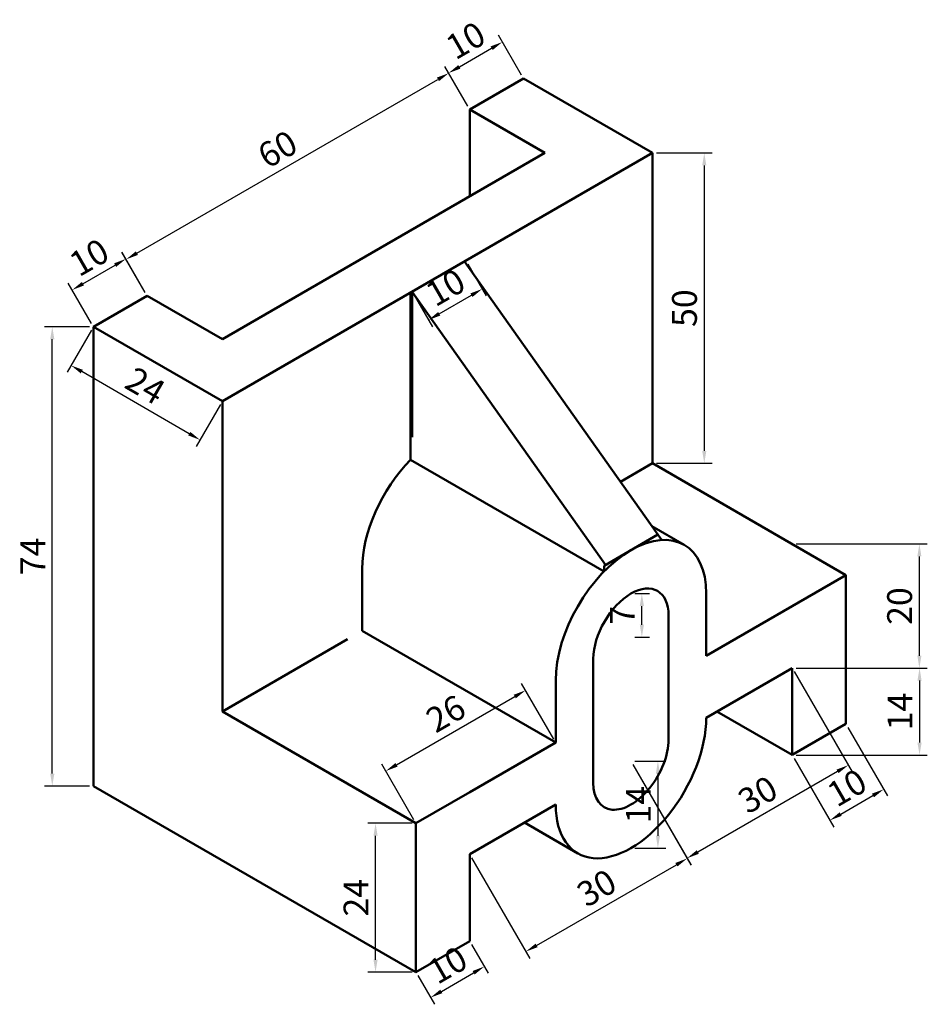
# Model space of a CAD drawing. Units: millimetres. Extents: x 109 to 256, y 55 to 213.
import ezdxf

# ---------------------------------------------------------------- set-up
doc = ezdxf.new("R2010")
doc.units = ezdxf.units.MM
doc.layers.add('M-DIMS', color=2, linetype='Continuous', lineweight=25)
doc.layers.add('M-OUTL', color=7, linetype='Continuous', lineweight=50)
doc.styles.get("Standard").update_dxf_attribs({"font": 'arial.ttf'})
doc.dimstyles.new('ISO-25', dxfattribs={"dimtxt": 4, "dimasz": 2, "dimexe": 1.25, "dimexo": 0.625, "dimtad": 1, "dimtxsty": 'Standard', "dimcen": 2.5, "dimadec": 0, "dimazin": 0, "dimtfac": 1, "dimtmove": 0, "dimatfit": 3, "dimfxl": 1, "dimarcsym": 0})

# ---------------------------------------------------------------- blocks, each defined once
blk = doc.blocks.new('*D1')
at = {"layer": 'Defpoints', "color": 0, "transparency": 16777216}
for p in [(121.32, 163.94), (117.73, 157.71), (142.11, 151.94)]:
    blk.add_point(p, dxfattribs=at)
at = {"layer": 'M-DIMS', "color": 0, "lineweight": -2, "transparency": 16777216}
for p, q in [((121.01, 163.4), (117.1, 156.63)), ((136.78, 146.71), (119.46, 156.71)), ((141.8, 151.4), (137.89, 144.63))]:
    blk.add_line(p, q, dxfattribs=at)
at = {"layer": 'M-DIMS', "color": 0, "transparency": 16777216}
for points in [[(119.63, 157), (119.29, 156.43), (117.73, 157.71)], [(136.95, 147), (136.61, 146.43), (138.51, 145.71)]]:
    blk.add_solid(points, dxfattribs=at)
at = {"layer": 'M-DIMS', "color": 0, "transparency": 16777216, "insert": (129.44, 154), "char_height": 4, "attachment_point": 5, "rotation": 330}
blk.add_mtext('24', dxfattribs=at)
blk = doc.blocks.new('*D2')
at = {"layer": 'Defpoints', "color": 0, "transparency": 16777216}
for p in [(126.56, 174.87), (129.98, 168.94), (121.32, 163.94)]:
    blk.add_point(p, dxfattribs=at)
at = {"layer": 'M-DIMS', "color": 0, "lineweight": -2, "transparency": 16777216}
for p, q in [((129.67, 169.48), (125.93, 175.96)), ((119.63, 170.87), (124.83, 173.87)), ((121.01, 164.48), (117.27, 170.96))]:
    blk.add_line(p, q, dxfattribs=at)
at = {"layer": 'M-DIMS', "color": 0, "transparency": 16777216}
for points in [[(124.66, 174.16), (124.99, 173.59), (126.56, 174.87)], [(119.47, 171.16), (119.8, 170.59), (117.9, 169.87)]]:
    blk.add_solid(points, dxfattribs=at)
at = {"layer": 'M-DIMS', "color": 0, "transparency": 16777216, "insert": (120.9, 174.68), "char_height": 4, "attachment_point": 5, "rotation": 30}
blk.add_mtext('10', dxfattribs=at)
blk = doc.blocks.new('*D3')
at = {"layer": 'Defpoints', "color": 0, "transparency": 16777216}
for p in [(178.56, 204.8), (181.95, 198.94), (129.98, 168.94)]:
    blk.add_point(p, dxfattribs=at)
at = {"layer": 'M-DIMS', "color": 0, "lineweight": -2, "transparency": 16777216}
for p, q in [((181.63, 199.48), (177.94, 205.88)), ((128.33, 175.8), (176.83, 203.8)), ((129.67, 169.48), (125.98, 175.88))]:
    blk.add_line(p, q, dxfattribs=at)
at = {"layer": 'M-DIMS', "color": 0, "transparency": 16777216}
for points in [[(176.67, 204.09), (177, 203.51), (178.56, 204.8)], [(128.17, 176.09), (128.5, 175.51), (126.6, 174.8)]]:
    blk.add_solid(points, dxfattribs=at)
at = {"layer": 'M-DIMS', "color": 0, "transparency": 16777216, "insert": (151.25, 192.11), "char_height": 4, "attachment_point": 5, "rotation": 30}
blk.add_mtext('60', dxfattribs=at)
blk = doc.blocks.new('*D4')
at = {"layer": 'Defpoints', "color": 0, "transparency": 16777216}
for p in [(187.21, 209.82), (190.61, 203.94), (181.95, 198.94)]:
    blk.add_point(p, dxfattribs=at)
at = {"layer": 'M-DIMS', "color": 0, "lineweight": -2, "transparency": 16777216}
for p, q in [((190.29, 204.48), (186.59, 210.9)), ((180.29, 205.82), (185.48, 208.82)), ((181.63, 199.48), (177.93, 205.9))]:
    blk.add_line(p, q, dxfattribs=at)
at = {"layer": 'M-DIMS', "color": 0, "transparency": 16777216}
for points in [[(185.31, 209.11), (185.65, 208.53), (187.21, 209.82)], [(180.12, 206.11), (180.45, 205.53), (178.55, 204.82)]]:
    blk.add_solid(points, dxfattribs=at)
at = {"layer": 'M-DIMS', "color": 0, "transparency": 16777216, "insert": (181.55, 209.63), "char_height": 4, "attachment_point": 5, "rotation": 30}
blk.add_mtext('10', dxfattribs=at)
blk = doc.blocks.new('*D5')
at = {"layer": 'Defpoints', "color": 0, "transparency": 16777216}
for p in [(211.39, 191.94), (211.39, 141.94), (219.74, 141.94)]:
    blk.add_point(p, dxfattribs=at)
at = {"layer": 'M-DIMS', "color": 0, "lineweight": -2, "transparency": 16777216}
for p, q in [((212.02, 191.94), (220.99, 191.94)), ((219.74, 189.94), (219.74, 143.94)), ((212.02, 141.94), (220.99, 141.94))]:
    blk.add_line(p, q, dxfattribs=at)
at = {"layer": 'M-DIMS', "color": 0, "transparency": 16777216}
for points in [[(219.4, 189.94), (220.07, 189.94), (219.74, 191.94)], [(219.4, 143.94), (220.07, 143.94), (219.74, 141.94)]]:
    blk.add_solid(points, dxfattribs=at)
at = {"layer": 'M-DIMS', "color": 0, "transparency": 16777216, "insert": (217.07, 166.94), "char_height": 4, "attachment_point": 5, "rotation": 90}
blk.add_mtext('50', dxfattribs=at)
blk = doc.blocks.new('*D6')
at = {"layer": 'Defpoints', "color": 0, "transparency": 16777216}
for p in [(233.91, 128.94), (254.39, 128.94), (233.91, 108.94)]:
    blk.add_point(p, dxfattribs=at)
at = {"layer": 'M-DIMS', "color": 0, "lineweight": -2, "transparency": 16777216}
for p, q in [((234.53, 128.94), (255.64, 128.94)), ((254.39, 110.94), (254.39, 126.94)), ((234.53, 108.94), (255.64, 108.94))]:
    blk.add_line(p, q, dxfattribs=at)
at = {"layer": 'M-DIMS', "color": 0, "transparency": 16777216}
for points in [[(254.06, 126.94), (254.72, 126.94), (254.39, 128.94)], [(254.06, 110.94), (254.72, 110.94), (254.39, 108.94)]]:
    blk.add_solid(points, dxfattribs=at)
at = {"layer": 'M-DIMS', "color": 0, "transparency": 16777216, "insert": (251.72, 118.94), "char_height": 4, "attachment_point": 5, "rotation": 90}
blk.add_mtext('20', dxfattribs=at)
blk = doc.blocks.new('*D7')
at = {"layer": 'Defpoints', "color": 0, "transparency": 16777216}
for p in [(233.91, 108.94), (233.91, 94.94), (254.42, 94.94)]:
    blk.add_point(p, dxfattribs=at)
at = {"layer": 'M-DIMS', "color": 0, "lineweight": -2, "transparency": 16777216}
for p, q in [((234.53, 108.94), (255.67, 108.94)), ((254.42, 106.94), (254.42, 96.94)), ((234.53, 94.94), (255.67, 94.94))]:
    blk.add_line(p, q, dxfattribs=at)
at = {"layer": 'M-DIMS', "color": 0, "transparency": 16777216}
for points in [[(254.08, 106.94), (254.75, 106.94), (254.42, 108.94)], [(254.08, 96.94), (254.75, 96.94), (254.42, 94.94)]]:
    blk.add_solid(points, dxfattribs=at)
at = {"layer": 'M-DIMS', "color": 0, "transparency": 16777216, "insert": (251.78, 101.94), "char_height": 4, "attachment_point": 5, "rotation": 90}
blk.add_mtext('14', dxfattribs=at)
blk = doc.blocks.new('*D8')
at = {"layer": 'Defpoints', "color": 0, "transparency": 16777216}
for p in [(166.78, 83.94), (173.29, 83.94), (173.29, 59.94)]:
    blk.add_point(p, dxfattribs=at)
at = {"layer": 'M-DIMS', "color": 0, "lineweight": -2, "transparency": 16777216}
for p, q in [((172.66, 83.94), (165.53, 83.94)), ((166.78, 61.94), (166.78, 81.94)), ((172.66, 59.94), (165.53, 59.94))]:
    blk.add_line(p, q, dxfattribs=at)
at = {"layer": 'M-DIMS', "color": 0, "transparency": 16777216}
for points in [[(166.45, 81.94), (167.11, 81.94), (166.78, 83.94)], [(166.45, 61.94), (167.11, 61.94), (166.78, 59.94)]]:
    blk.add_solid(points, dxfattribs=at)
at = {"layer": 'M-DIMS', "color": 0, "transparency": 16777216, "insert": (164.15, 71.94), "char_height": 4, "attachment_point": 5, "rotation": 90}
blk.add_mtext('24', dxfattribs=at)
blk = doc.blocks.new('*D9')
at = {"layer": 'Defpoints', "color": 0, "transparency": 16777216}
for p in [(181.95, 64.94), (184.31, 60.86), (173.29, 59.94)]:
    blk.add_point(p, dxfattribs=at)
at = {"layer": 'M-DIMS', "color": 0, "lineweight": -2, "transparency": 16777216}
for p, q in [((182.26, 64.4), (184.93, 59.77)), ((173.6, 59.4), (176.27, 54.77)), ((177.38, 56.86), (182.57, 59.86))]:
    blk.add_line(p, q, dxfattribs=at)
at = {"layer": 'M-DIMS', "color": 0, "transparency": 16777216}
for points in [[(182.41, 60.14), (182.74, 59.57), (184.31, 60.86)], [(177.21, 57.14), (177.54, 56.57), (175.65, 55.86)]]:
    blk.add_solid(points, dxfattribs=at)
at = {"layer": 'M-DIMS', "color": 0, "transparency": 16777216, "insert": (178.64, 60.67), "char_height": 4, "attachment_point": 5, "rotation": 30}
blk.add_mtext('10', dxfattribs=at)
blk = doc.blocks.new('*D10')
at = {"layer": 'Defpoints', "color": 0, "transparency": 16777216}
for p in [(207.93, 93.94), (181.95, 78.94), (216.98, 78.27)]:
    blk.add_point(p, dxfattribs=at)
at = {"layer": 'M-DIMS', "color": 0, "lineweight": -2, "transparency": 16777216}
for p, q in [((208.24, 93.4), (217.6, 77.18)), ((182.26, 78.4), (191.62, 62.18)), ((192.73, 64.27), (215.25, 77.27))]:
    blk.add_line(p, q, dxfattribs=at)
at = {"layer": 'M-DIMS', "color": 0, "transparency": 16777216}
for points in [[(215.08, 77.55), (215.41, 76.98), (216.98, 78.27)], [(192.56, 64.55), (192.9, 63.98), (191, 63.27)]]:
    blk.add_solid(points, dxfattribs=at)
at = {"layer": 'M-DIMS', "color": 0, "transparency": 16777216, "insert": (202.65, 73.08), "char_height": 4, "attachment_point": 5, "rotation": 30}
blk.add_mtext('30', dxfattribs=at)
blk = doc.blocks.new('*D11')
at = {"layer": 'Defpoints', "color": 0, "transparency": 16777216}
for p in [(233.91, 108.94), (207.93, 93.94), (216.96, 78.3)]:
    blk.add_point(p, dxfattribs=at)
at = {"layer": 'M-DIMS', "color": 0, "lineweight": -2, "transparency": 16777216}
for p, q in [((234.22, 108.4), (243.56, 92.22)), ((208.24, 93.4), (217.58, 77.22)), ((241.2, 92.3), (218.69, 79.3))]:
    blk.add_line(p, q, dxfattribs=at)
at = {"layer": 'M-DIMS', "color": 0, "transparency": 16777216}
for points in [[(241.04, 92.59), (241.37, 92.02), (242.94, 93.3)], [(218.52, 79.59), (218.85, 79.02), (216.96, 78.3)]]:
    blk.add_solid(points, dxfattribs=at)
at = {"layer": 'M-DIMS', "color": 0, "transparency": 16777216, "insert": (228.61, 88.12), "char_height": 4, "attachment_point": 5, "rotation": 30}
blk.add_mtext('30', dxfattribs=at)
blk = doc.blocks.new('*D12')
at = {"layer": 'Defpoints', "color": 0, "transparency": 16777216}
for p in [(242.57, 99.94), (233.91, 94.94), (248.64, 89.42)]:
    blk.add_point(p, dxfattribs=at)
at = {"layer": 'M-DIMS', "color": 0, "lineweight": -2, "transparency": 16777216}
for p, q in [((242.88, 99.4), (249.27, 88.34)), ((234.22, 94.4), (240.61, 83.34)), ((241.72, 85.42), (246.91, 88.42))]:
    blk.add_line(p, q, dxfattribs=at)
at = {"layer": 'M-DIMS', "color": 0, "transparency": 16777216}
for points in [[(246.74, 88.71), (247.08, 88.13), (248.64, 89.42)], [(241.55, 85.71), (241.88, 85.13), (239.98, 84.42)]]:
    blk.add_solid(points, dxfattribs=at)
at = {"layer": 'M-DIMS', "color": 0, "transparency": 16777216, "insert": (242.98, 89.23), "char_height": 4, "attachment_point": 5, "rotation": 30}
blk.add_mtext('10', dxfattribs=at)
blk = doc.blocks.new('*D13')
at = {"layer": 'Defpoints', "color": 0, "transparency": 16777216}
for p in [(207.93, 93.94), (207.93, 79.94), (212.27, 79.94)]:
    blk.add_point(p, dxfattribs=at)
at = {"layer": 'M-DIMS', "color": 0, "lineweight": -2, "transparency": 16777216}
for p, q in [((208.55, 93.94), (213.52, 93.94)), ((212.27, 91.94), (212.27, 81.94)), ((208.55, 79.94), (213.52, 79.94))]:
    blk.add_line(p, q, dxfattribs=at)
at = {"layer": 'M-DIMS', "color": 0, "transparency": 16777216}
for points in [[(211.94, 91.94), (212.61, 91.94), (212.27, 93.94)], [(211.94, 81.94), (212.61, 81.94), (212.27, 79.94)]]:
    blk.add_solid(points, dxfattribs=at)
at = {"layer": 'M-DIMS', "color": 0, "transparency": 16777216, "insert": (209.64, 86.94), "char_height": 4, "attachment_point": 5, "rotation": 90}
blk.add_mtext('14', dxfattribs=at)
blk = doc.blocks.new('*D14')
at = {"layer": 'Defpoints', "color": 0, "transparency": 16777216}
for p in [(207.93, 120.94), (209.68, 120.94), (207.93, 113.94)]:
    blk.add_point(p, dxfattribs=at)
at = {"layer": 'M-DIMS', "color": 0, "lineweight": -2, "transparency": 16777216}
for p, q in [((208.55, 120.94), (210.93, 120.94)), ((209.68, 115.94), (209.68, 118.94)), ((208.55, 113.94), (210.93, 113.94))]:
    blk.add_line(p, q, dxfattribs=at)
at = {"layer": 'M-DIMS', "color": 0, "transparency": 16777216}
for points in [[(209.35, 118.94), (210.02, 118.94), (209.68, 120.94)], [(209.35, 115.94), (210.02, 115.94), (209.68, 113.94)]]:
    blk.add_solid(points, dxfattribs=at)
at = {"layer": 'M-DIMS', "color": 0, "transparency": 16777216, "insert": (207.06, 117.44), "char_height": 4, "attachment_point": 5, "rotation": 90}
blk.add_mtext('7', dxfattribs=at)
blk = doc.blocks.new('*D15')
at = {"layer": 'Defpoints', "color": 0, "transparency": 16777216}
for p in [(181.33, 174.59), (183.96, 170.03), (172.67, 169.59)]:
    blk.add_point(p, dxfattribs=at)
at = {"layer": 'M-DIMS', "color": 0, "lineweight": -2, "transparency": 16777216}
for p, q in [((181.64, 174.05), (184.59, 168.95)), ((172.98, 169.05), (175.93, 163.95)), ((177.03, 166.03), (182.23, 169.03))]:
    blk.add_line(p, q, dxfattribs=at)
at = {"layer": 'M-DIMS', "color": 0, "transparency": 16777216}
for points in [[(182.06, 169.32), (182.4, 168.74), (183.96, 170.03)], [(176.87, 166.32), (177.2, 165.74), (175.3, 165.03)]]:
    blk.add_solid(points, dxfattribs=at)
at = {"layer": 'M-DIMS', "color": 0, "transparency": 16777216, "insert": (178.3, 169.84), "char_height": 4, "attachment_point": 5, "rotation": 30}
blk.add_mtext('10', dxfattribs=at)
blk = doc.blocks.new('*D16')
at = {"layer": 'Defpoints', "color": 0, "transparency": 16777216}
for p in [(190.94, 105.36), (195.8, 96.94), (173.29, 83.94)]:
    blk.add_point(p, dxfattribs=at)
at = {"layer": 'M-DIMS', "color": 0, "lineweight": -2, "transparency": 16777216}
for p, q in [((195.49, 97.48), (190.32, 106.44)), ((170.16, 93.36), (189.21, 104.36)), ((172.97, 84.48), (167.8, 93.44))]:
    blk.add_line(p, q, dxfattribs=at)
at = {"layer": 'M-DIMS', "color": 0, "transparency": 16777216}
for points in [[(189.05, 104.65), (189.38, 104.07), (190.94, 105.36)], [(169.99, 93.65), (170.33, 93.07), (168.43, 92.36)]]:
    blk.add_solid(points, dxfattribs=at)
at = {"layer": 'M-DIMS', "color": 0, "transparency": 16777216, "insert": (178.35, 101.17), "char_height": 4, "attachment_point": 5, "rotation": 30}
blk.add_mtext('26', dxfattribs=at)
blk = doc.blocks.new('*D17')
at = {"layer": 'Defpoints', "color": 0, "transparency": 16777216}
for p in [(114.7, 163.94), (121.32, 163.94), (121.32, 89.94)]:
    blk.add_point(p, dxfattribs=at)
at = {"layer": 'M-DIMS', "color": 0, "lineweight": -2, "transparency": 16777216}
for p, q in [((120.7, 163.94), (113.45, 163.94)), ((114.7, 91.94), (114.7, 161.94)), ((120.7, 89.94), (113.45, 89.94))]:
    blk.add_line(p, q, dxfattribs=at)
at = {"layer": 'M-DIMS', "color": 0, "transparency": 16777216}
for points in [[(114.37, 161.94), (115.04, 161.94), (114.7, 163.94)], [(114.37, 91.94), (115.04, 91.94), (114.7, 89.94)]]:
    blk.add_solid(points, dxfattribs=at)
at = {"layer": 'M-DIMS', "color": 0, "transparency": 16777216, "insert": (112.08, 126.94), "char_height": 4, "attachment_point": 5, "rotation": 90}
blk.add_mtext('74', dxfattribs=at)

msp = doc.modelspace()

# ---------------------------------------------------------------- linework, layer by layer
at = {"layer": 'M-OUTL'}
for p, q in [((181.946, 198.944), (190.606, 203.944)), ((190.606, 203.944), (211.391, 191.944)), ((194.07, 191.944), (181.946, 198.944)), ((181.946, 198.944), (181.946, 184.944)), ((142.109, 161.944), (194.07, 191.944)), ((211.391, 191.944), (142.109, 151.944)), ((211.391, 191.944), (211.391, 141.944)), ((181.099, 174.454), (212.006, 130.834)), ((142.109, 151.944), (176.75, 171.944)), ((121.324, 163.944), (129.984, 168.944)), ((129.984, 168.944), (142.109, 161.944)), ((172.42, 142.52), (172.42, 169.444)), ((172.67, 169.588), (203.847, 125.588)), ((172.67, 169.588), (172.67, 146.152)), ((121.324, 89.944), (121.324, 163.944)), ((121.324, 163.944), (142.109, 151.944)), ((142.109, 151.944), (142.109, 101.944)), ((172.42, 142.52), (203.597, 124.52)), ((206.241, 138.971), (211.391, 141.944)), ((211.391, 141.944), (242.568, 123.944)), ((211.299, 131.796), (216.5, 128.793)), ((212.257, 130.444), (203.597, 125.444)), ((212.006, 130.834), (212.893, 129.583)), ((203.597, 125.444), (203.597, 124.52)), ((164.625, 114.944), (164.625, 124.944)), ((242.568, 123.944), (220.051, 110.944)), ((242.568, 99.944), (242.568, 123.944)), ((220.051, 120.944), (220.051, 110.944)), ((213.989, 117.444), (213.989, 97.444)), ((195.802, 96.944), (164.625, 114.944)), ((142.109, 101.944), (162.28, 113.589)), ((142.109, 101.944), (162.28, 113.589)), ((201.865, 110.444), (201.865, 90.444)), ((220.051, 100.944), (233.907, 108.944)), ((233.907, 108.944), (233.907, 94.944)), ((195.802, 96.944), (195.802, 106.944)), ((142.109, 101.944), (173.286, 83.944)), ((233.907, 94.944), (221.783, 101.944)), ((233.907, 94.944), (242.568, 99.944)), ((181.946, 88.944), (195.802, 96.944)), ((121.324, 89.944), (173.286, 59.944)), ((173.286, 83.944), (181.946, 88.944)), ((181.946, 78.944), (195.802, 86.944)), ((173.286, 59.944), (173.286, 83.944)), ((190.78, 84.044), (199.353, 79.094)), ((181.946, 64.944), (181.946, 78.944)), ((173.286, 59.944), (181.946, 64.944))]:
    msp.add_line(p, q, dxfattribs=at)
for centre, major_axis, start_param, end_param in [((176.75, 131.944), (8.573, 14.849), 1.1506054, 2.3561945), ((207.927, 113.944), (-8.573, -14.849), 2.3561945, 5.4977871), ((207.927, 113.944), (-4.287, -7.425), 2.3561945, 5.4977871), ((207.927, 93.944), (-8.573, -14.849), 5.4977871, 8.6393798), ((207.927, 93.944), (-4.287, -7.425), 5.4977871, 8.6393798)]:
    msp.add_ellipse(centre, major_axis=major_axis, ratio=0.5773503, start_param=start_param, end_param=end_param, dxfattribs=at)

# ---------------------------------------------------------------- dimensions: what is measured, and where the dimension line sits
at = {"layer": 'M-DIMS'}
for p1, p2, distance, picture, middle in [((181.946, 198.944), (190.606, 203.944), 6.785, '*D4', (181.55, 209.63)), ((129.984, 168.944), (181.946, 198.944), 6.763, '*D3', (151.25, 192.111)), ((121.324, 163.944), (129.984, 168.944), 6.849, '*D2', (120.896, 174.685)), ((172.67, 169.588), (181.33, 174.588), -5.263, '*D15', (178.298, 169.84)), ((142.109, 151.944), (121.324, 163.944), 7.193, '*D1', (129.437, 153.995)), ((233.907, 108.944), (207.927, 93.944), 18.059, '*D11', (228.612, 88.115)), ((173.286, 83.944), (195.802, 96.944), 9.717, '*D16', (178.352, 101.169)), ((233.907, 94.944), (242.568, 99.944), -12.151, '*D12', (242.979, 89.23)), ((181.946, 78.944), (207.927, 93.944), -18.104, '*D10', (202.654, 73.076)), ((173.286, 59.944), (181.946, 64.944), -4.72, '*D9', (178.642, 60.666))]:
    dim = msp.add_aligned_dim(p1=p1, p2=p2, distance=distance, dimstyle='ISO-25', override={"dimclrd": 0, "dimclre": 0, "dimclrt": 0}, dxfattribs=at)
    dim.commit()
    dim.dimension.update_dxf_attribs({"geometry": picture, "text_midpoint": middle})
for base, p1, p2, picture, middle in [((219.736, 141.944), (211.391, 191.944), (211.391, 141.944), '*D5', (217.069, 166.944)), ((114.704, 163.944), (121.324, 89.944), (121.324, 163.944), '*D17', (112.079, 126.944)), ((254.39, 128.944), (233.907, 108.944), (233.907, 128.944), '*D6', (251.723, 118.944)), ((209.684, 120.944), (207.927, 113.944), (207.927, 120.944), '*D14', (207.059, 117.444)), ((254.417, 94.944), (233.907, 108.944), (233.907, 94.944), '*D7', (251.784, 101.944)), ((212.274, 79.944), (207.927, 93.944), (207.927, 79.944), '*D13', (209.64, 86.944)), ((166.781, 83.944), (173.286, 59.944), (173.286, 83.944), '*D8', (164.148, 71.944))]:
    dim = msp.add_linear_dim(base=base, p1=p1, p2=p2, angle=90, dimstyle='ISO-25', override={"dimclrd": 0, "dimclre": 0, "dimclrt": 0}, dxfattribs=at)
    dim.commit()
    dim.dimension.update_dxf_attribs({"geometry": picture, "text_midpoint": middle})

doc.saveas('drawing.dxf')
